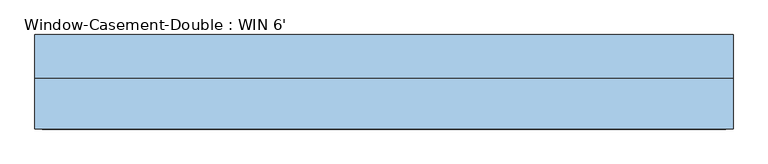
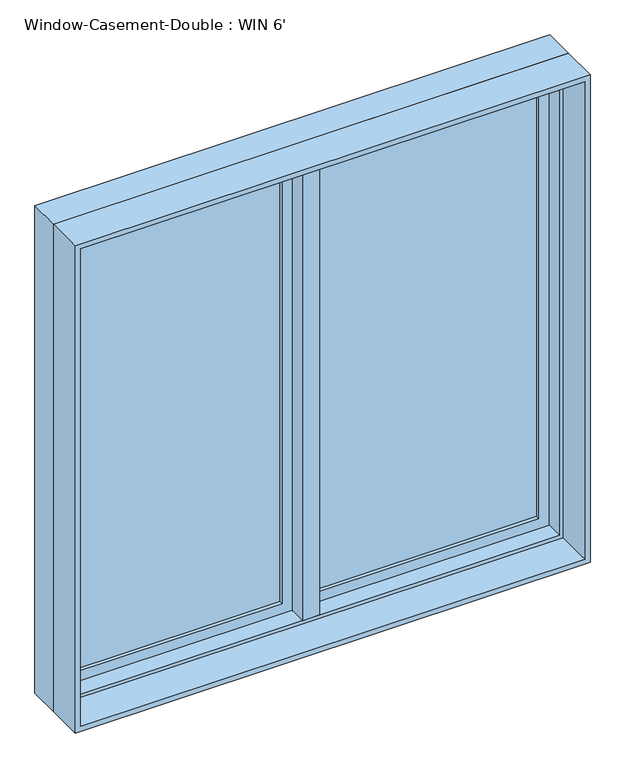
"""IFC4 building model written with IfcOpenShell, lengths in millimetres: window geometry, Window-Casement-Double : WIN 6'."""

from ifc_helpers import new_model, si_unit, frame, origin, place, context, project, spatial, polyline, outline, extrude, faceted_brep, source, transform, mapped, element, save


def window_casement_double_win_6_ce442eab(model_context):
    return source(origin(), model_context, "Body", "SolidModel", [
        faceted_brep([(9.525, 133.35, 2730.5), (-9.525, 133.35, 2730.5), (-9.525, 82.55, 2730.5), (9.525, 82.55, 2730.5), (9.525, 133.35, 927.1), (9.525, 82.55, 927.1), (-9.525, 82.55, 927.1), (-9.525, 133.35, 927.1), (-9.525, 82.55, 946.15), (-9.525, 82.55, 2711.45), (-30.1625, 82.55, 946.15), (-30.1625, 82.55, 2711.45), (-30.1625, 19.05, 946.15), (-30.1625, 19.05, 2711.45), (30.1625, 19.05, 946.15), (30.1625, 19.05, 2711.45), (30.1625, 82.55, 946.15), (30.1625, 82.55, 2711.45), (9.525, 82.55, 946.15), (9.525, 82.55, 2711.45)], [[[0, 1, 2, 3]], [[4, 5, 6, 7]], [[1, 0, 4, 7]], [[2, 1, 7, 6, 8, 9]], [[9, 8, 10, 11]], [[11, 10, 12, 13]], [[13, 12, 14, 15]], [[15, 14, 16, 17]], [[17, 16, 18, 19]], [[0, 3, 19, 18, 5, 4]], [[18, 8, 6, 5]], [[9, 19, 3, 2]], [[8, 18, 16, 14, 12, 10]], [[19, 9, 11, 13, 15, 17]]]),
        extrude(outline(polyline([(-66.675, 114.3), (-66.675, 107.95), (-844.55, 107.95), (-844.55, 114.3), (-66.675, 114.3)])), frame((0.0, 0.0, 984.25), z_axis=(0.0, 0.0, 1.0), x_axis=(1.0, 0.0, 0.0)), (0.0, 0.0, 1.0), 1689.1),
        extrude(outline(polyline([(-844.55, 95.25), (-844.55, 101.6), (-66.675, 101.6), (-66.675, 95.25), (-844.55, 95.25)])), frame((0.0, 0.0, 984.25), z_axis=(0.0, 0.0, 1.0), x_axis=(1.0, 0.0, 0.0)), (0.0, 0.0, 1.0), 1689.1),
        extrude(outline(polyline([(844.55, 114.3), (844.55, 107.95), (66.675, 107.95), (66.675, 114.3), (844.55, 114.3)])), frame((0.0, 0.0, 984.25), z_axis=(0.0, 0.0, 1.0), x_axis=(1.0, 0.0, 0.0)), (0.0, 0.0, 1.0), 1689.1),
        extrude(outline(polyline([(66.675, 95.25), (66.675, 101.6), (844.55, 101.6), (844.55, 95.25), (66.675, 95.25)])), frame((0.0, 0.0, 984.25), z_axis=(0.0, 0.0, 1.0), x_axis=(1.0, 0.0, 0.0)), (0.0, 0.0, 1.0), 1689.1),
        extrude(outline(polyline([(2730.5, -901.7), (927.1, -901.7), (927.1, -9.525), (2730.5, -9.525), (2730.5, -901.7)]), holes=[polyline([(2673.35, -66.675), (984.25, -66.675), (984.25, -844.55), (2673.35, -844.55), (2673.35, -66.675)])]), frame((0.0, 82.55, 0.0), z_axis=(0.0, 1.0, 0.0), x_axis=(0.0, 0.0, 1.0)), (0.0, 0.0, 1.0), 44.45),
        extrude(outline(polyline([(927.1, 901.7), (2730.5, 901.7), (2730.5, 9.525), (927.1, 9.525), (927.1, 901.7)]), holes=[polyline([(984.25, 66.675), (2673.35, 66.675), (2673.35, 844.55), (984.25, 844.55), (984.25, 66.675)])]), frame((0.0, 82.55, 0.0), z_axis=(0.0, 1.0, 0.0), x_axis=(0.0, 0.0, 1.0)), (0.0, 0.0, 1.0), 44.45),
        extrude(outline(polyline([(2743.2, -914.4), (914.4, -914.4), (914.4, 914.4), (2743.2, 914.4), (2743.2, -914.4)]), holes=[polyline([(2724.15, 895.35), (933.45, 895.35), (933.45, -895.35), (2724.15, -895.35), (2724.15, 895.35)])]), frame((0.0, -114.3, 0.0), z_axis=(0.0, 1.0, 0.0), x_axis=(0.0, 0.0, 1.0)), (0.0, 0.0, 1.0), 133.35),
        faceted_brep([(882.65, 82.55, 2711.45), (882.65, 19.05, 2711.45), (-882.65, 19.05, 2711.45), (-882.65, 82.55, 2711.45), (901.7, 133.35, 2730.5), (901.7, 82.55, 2730.5), (-901.7, 82.55, 2730.5), (-901.7, 133.35, 2730.5), (914.4, 19.05, 2743.2), (914.4, 133.35, 2743.2), (-914.4, 133.35, 2743.2), (-914.4, 19.05, 2743.2), (-882.65, 19.05, 946.15), (-882.65, 82.55, 946.15), (-901.7, 82.55, 927.1), (-901.7, 133.35, 927.1), (-914.4, 133.35, 914.4), (-914.4, 19.05, 914.4), (882.65, 19.05, 946.15), (882.65, 82.55, 946.15), (901.7, 82.55, 927.1), (901.7, 133.35, 927.1), (914.4, 133.35, 914.4), (914.4, 19.05, 914.4)], [[[0, 1, 2, 3]], [[4, 5, 6, 7]], [[8, 9, 10, 11]], [[3, 2, 12, 13]], [[7, 6, 14, 15]], [[11, 10, 16, 17]], [[13, 12, 18, 19]], [[15, 14, 20, 21]], [[17, 16, 22, 23]], [[11, 17, 23, 8], [1, 18, 12, 2]], [[19, 18, 1, 0]], [[5, 20, 14, 6], [3, 13, 19, 0]], [[21, 20, 5, 4]], [[23, 22, 9, 8]], [[9, 22, 16, 10], [7, 15, 21, 4]]]),
    ])


if __name__ == "__main__":
    model = new_model("IFC4")
    model_context = context("Model", 3, world=origin())
    ifc_project = project(units=[si_unit("LENGTHUNIT", "METRE", prefix="MILLI")], contexts=[model_context])
    site = spatial("IfcSite", under=ifc_project)
    building = spatial("IfcBuilding", under=site)
    placement = place(None, origin())
    window_casement_double_win_6_shape = window_casement_double_win_6_ce442eab(model_context)
    element("IfcWindow", 1, ObjectType="Window-Casement-Double : WIN 6'", at=placement, inside=building, context=model_context, shape_type="MappedRepresentation", body=[
        mapped(window_casement_double_win_6_shape, transform((0.0, 0.0, 0.0), x_axis=(1.0, 0.0, 0.0), y_axis=(0.0, 1.0, 0.0), z_axis=(0.0, 0.0, 1.0))),
    ])
    save(model, "model.ifc")

# Revit data of these elements
# Type "Window-Casement-Double : WIN 6'"
#   Type Mark = "19"
#   Fire Rating = "0.5h"
#   Assembly Code = "B2020100"
#   Analytic Construction = "Double glazing - domestic"
#   Frame Extension [instance default] = 0' - 0 1/4"
#   Window Inset [instance default] = 0' - 0"
#   Wall Thickness [instance default] = 0' - 6"
#   Interior Wall Closure [instance default] = 0' - 2 1/4"
#   Half Width = 3' - 0"
#   Visual Light Transmittance = 0.81
#   Thermal Resistance (R) = 1.8146 (h·ft²·°F)/BTU
#   Solar Heat Gain Coefficient = 0.76
#   Rough Width = 6' - 0 1/2"
#   Rough Height = 6' - 0 1/2"
#   Height = 6' - 0"
#   Heat Transfer Coefficient (U) = 0.5511 BTU/(h·ft²·°F)
#   Exterior Wall Closure [instance default] = 0' - 1 1/4"
#   Extension Jamb [instance default] = 0' - 2 1/4"
#   Default Sill Height = 3' - 0"
#   Width = 6' - 0"
#   Muntin Visibility = yes
#   Interior Trim Visibility [instance default] = yes
#   Exterior Trim Visibility [instance default] = yes
#   Extension Jamb Visibility [instance default] = yes
#   Interior Trim Material = Wood - Stained
#   Muntin Pattern = Muntin Pattern_2x2 : Muntin Pattern_2x2
#   Interior Trim = Trim-Window-Interior-Flat : Picture Frame
#   Interior Frame Material = Wood - Stained
#   Glass Panel Material = Glass
#   Exterior Trim Material = Clad - White
#   Exterior Trim = Trim-Window-Exterior-Flat : with Sill
#   Exterior Frame Material = Clad - White
#   Wall Closure = (empty or 0)
# Element 1 (IfcWindow, "Window-Casement-Double : WIN 6'")
#   Wall Thickness = 0' - 9"
#   Extension Jamb = 0' - 5 1/4"
#   Materials on its faces: "Wood - Stained", "Glass", "Clad - White"
# Materials
#   "Wood - Stained": class "Wood", colour RGB 224 178 126, transparency 0, Cost = 0
#   "Glass": class "Glass", colour RGB 0 128 192, transparency 0.75, Description = "Soda Lime Glass", Cost = 0
#   "Clad - White": class "Wood", colour RGB 242 242 238, transparency 0, Cost = 0
